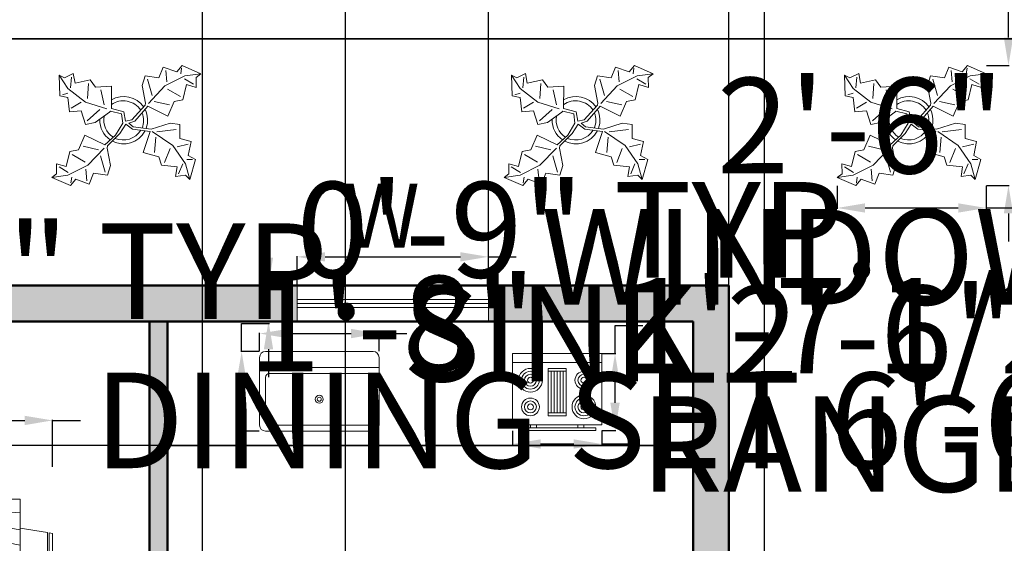
# Model space of a CAD drawing. Units: inches. Extents: x -166 to 1001, y 0 to 688.
# Tile 9 of 11: x 361 to 608, y 419 to 551. Entities that reach past the tile are written whole.
import ezdxf

# ---------------------------------------------------------------- set-up
doc = ezdxf.new("R2010")
doc.units = ezdxf.units.IN
doc.header["$MEASUREMENT"] = 0
for name, color, linetype, lineweight in [('A-ANNO-DIMS', 1, 'Continuous', 18), ('A-ANNO-TEXT', 2, 'Continuous', 25), ('A-EQPM', 11, 'Continuous', 18), ('A-FLOR-CASE', 32, 'Continuous', 25), ('A-FLOR-FIXT', 11, 'Continuous', 18), ('A-GLAZ', 130, 'Continuous', 18), ('A-WALL-PATT', 5, 'Continuous', 13), ('C-SITE-WALL', 250, 'Continuous', 35), ('FURNITURE', 11, 'Continuous', 18), ('TREES', 80, 'Continuous', 13), ('WALLS', 250, 'Continuous', 50)]:
    doc.layers.add(name, color=color, linetype=linetype, lineweight=lineweight)
doc.styles.get("Standard").update_dxf_attribs({"font": 'arial.ttf'})
doc.dimstyles.get("Standard").update_dxf_attribs({"dimtxt": 24, "dimasz": 7, "dimexe": 0.18, "dimexo": 0.0625, "dimgap": 0.09, "dimtad": 0, "dimtih": 1, "dimtoh": 1, "dimdec": 0, "dimzin": 0, "dimdsep": 46, "dimlunit": 3, "dimtxsty": 'Standard', "dimcen": 0.09, "dimadec": 0, "dimazin": 0, "dimtfac": 1, "dimtdec": 0, "dimtofl": 0, "dimtmove": 0, "dimatfit": 3, "dimfxl": 1, "dimtolj": 1, "dimtzin": 0, "dimarcsym": 0})

# ---------------------------------------------------------------- blocks, each defined once
blk = doc.blocks.new('Sink-single - 30 in top')
blk.add_line((-15, -3.999996), (15, -3.999996))
for points in [[(-13.5, 0), (13.5, 0)], [(-15, -18.499996), (-15, -1.5)], [(15, -1.5), (15, -18.499996)], [(-13.5, -17.499996), (-13.5, -6.499996)], [(-12.5, -5.499996), (12.5, -5.499996)], [(13.5, -6.499996), (13.5, -17.499996)], [(12.5, -18.499996), (-12.5, -18.499996)], [(13.5, -19.999996), (-13.5, -19.999996)]]:
    blk.add_lwpolyline(points)
for radius in [1, 0.5]:
    blk.add_circle((0, -11.999996), radius)
for centre, radius, start, end in [((-13.5, -1.5), 1.5, 90, 180), ((13.5, -1.5), 1.5, 0, 90), ((-12.5, -6.499996), 1, 90, 180), ((12.5, -6.499996), 1, 0, 90), ((-13.5, -18.499996), 1.5, 180, 270), ((-12.5, -17.499996), 1, 180, 270), ((12.5, -17.499996), 1, 270, 0), ((13.5, -18.499996), 1.5, 270, 0)]:
    blk.add_arc(centre, radius, start, end)
blk = doc.blocks.new('Range-Oven - 30 in top')
for p, q in [((0, -3), (30, -3)), ((12, -6), (18, -6)), ((13, -20), (13, -6)), ((14, -6), (14, -20)), ((15, -20), (15, -6)), ((16, -6), (16, -20)), ((17, -20), (17, -6)), ((18, -20), (12, -20)), ((6, -24), (6, -25)), ((8, -25), (8, -24)), ((22, -25), (22, -24)), ((24, -24), (24, -25))]:
    blk.add_line(p, q)
for points in [[(0, -24), (0, 0), (30, 0), (30, -24)], [(12, -21), (12, -5), (18, -5), (18, -21)], [(2, -26), (2, -25), (28, -25), (28, -26)]]:
    blk.add_lwpolyline(points, close=True)
for centre, radius in [((6, -9), 4), ((6, -9), 3), ((24, -9), 3), ((6, -9), 2), ((6, -9), 1), ((24, -9), 2), ((24, -9), 1), ((6, -18), 3), ((6, -18), 2), ((24, -18), 4), ((24, -18), 3), ((24, -18), 2), ((6, -18), 1), ((24, -18), 1)]:
    blk.add_circle(centre, radius)
blk = doc.blocks.new('Dining Set - 36 x 72 in.')
for p, q in [((-22.2343, 26.00059), (-23.4847, 17.99762)), ((-22.2304, 26), (-5.7608, 26)), ((-22, 27.5), (-22.1562, 26.50042)), ((-5.8416, 26.5), (-22.1534, 26.5)), ((-22, 27.5), (-6, 27.5)), ((-5.8437, 26.49966), (-6, 27.5)), ((-4.5152, 17.99762), (-5.7655, 25.99926)), ((5.7657, 26.00059), (4.5153, 17.99762)), ((5.7696, 26), (22.2392, 26)), ((6, 27.5), (5.8438, 26.50042)), ((22.1584, 26.5), (5.8466, 26.5)), ((6, 27.5), (22, 27.5)), ((22.1563, 26.49966), (22, 27.5)), ((23.4848, 17.99762), (22.2345, 25.99926)), ((36, 18), (-36, 18)), ((-36, 18), (-36, -18)), ((36, -18), (36, 18)), ((-44.0006, 8.23428), (-35.9976, 9.48474)), ((44.0006, 8.23428), (35.9976, 9.48474)), ((-45.5, 8), (-44.5004, 8.15617)), ((-45.5, 8), (-45.5, -8)), ((-44.5, -8.15843), (-44.5, 8.15338)), ((-44, 8.23041), (-44, -8.23915)), ((44, 8.23041), (44, -8.23915)), ((44.5, -8.15843), (44.5, 8.15338)), ((45.5, 8), (44.5005, 8.15617)), ((45.5, 8), (45.5, -8)), ((-44.4997, -8.15631), (-45.5, -8)), ((-35.9976, -9.48476), (-43.9993, -8.2345)), ((35.9976, -9.48476), (43.9993, -8.2345)), ((44.4997, -8.15631), (45.5, -8)), ((-36, -18), (36, -18)), ((-22.2343, -26.0006), (-23.4847, -17.99762)), ((-4.5152, -17.99762), (-5.7655, -25.99928)), ((5.7657, -26.0006), (4.5153, -17.99762)), ((23.4848, -17.99762), (22.2345, -25.99928)), ((-22.2304, -26), (-5.7608, -26)), ((-22, -27.5), (-22.1562, -26.50044)), ((-5.8416, -26.5), (-22.1534, -26.5)), ((-22, -27.5), (-6, -27.5)), ((-5.8437, -26.49967), (-6, -27.5)), ((5.7696, -26), (22.2392, -26)), ((6, -27.5), (5.8438, -26.50044)), ((22.1584, -26.5), (5.8466, -26.5)), ((6, -27.5), (22, -27.5)), ((22.1563, -26.49967), (22, -27.5))]:
    blk.add_line(p, q)
for points in [[(-36, 15), (-31.1772, 14.97754), (-26.8079, 14.91406), (-22.8538, 14.81543), (-19.276, 14.6875), (-16.0362, 14.53613), (-13.0957, 14.36718), (-10.4159, 14.18652), (-7.9583, 14), (-5.6904, 13.81315), (-3.6035, 13.63021), (-1.6954, 13.45508), (0.0365, 13.29166), (1.5945, 13.14388), (2.9811, 13.01562), (4.1988, 12.9108), (5.25, 12.83333), (6.1393, 12.78613), (6.8802, 12.76823), (7.4883, 12.77767), (7.9792, 12.8125), (8.3685, 12.87077), (8.6719, 12.95052), (8.9049, 13.0498), (9.0833, 13.16666), (9.2205, 13.29899), (9.3216, 13.44401), (9.3895, 13.59879), (9.4271, 13.76041), (9.4373, 13.92594), (9.4232, 14.09245), (9.3875, 14.257), (9.3333, 14.41666), (9.2638, 14.56917), (9.1836, 14.71484), (9.0975, 14.85465), (9.0104, 14.98958), (8.9272, 15.1206), (8.8529, 15.2487), (8.7922, 15.37483), (8.75, 15.5), (8.7305, 15.62467), (8.7344, 15.74739), (8.7617, 15.86621), (8.8125, 15.97916), (8.8867, 16.08431), (8.9844, 16.17968), (9.1055, 16.26334), (9.25, 16.33333), (9.4189, 16.38802), (9.6172, 16.42708), (9.8506, 16.45052), (10.125, 16.45833), (10.4463, 16.45052), (10.8203, 16.42708), (11.2529, 16.38802), (11.75, 16.33333), (12.3184, 16.26318), (12.9694, 16.17838), (13.7151, 16.07991), (14.5677, 15.96875), (15.5395, 15.84586), (16.6426, 15.71224), (17.8893, 15.56884), (19.2917, 15.41666), (20.859, 15.25667), (22.5879, 15.08984), (24.4721, 14.91715), (26.5052, 14.73958), (28.6809, 14.5581), (30.9929, 14.3737), (33.4347, 14.18733), (36, 14)], [(-36, 10), (-28.9766, 10.14274), (-23.1725, 10.20442), (-18.4241, 10.19775), (-14.5677, 10.13541), (-11.4399, 10.03011), (-8.877, 9.89453), (-6.7154, 9.74137), (-4.7917, 9.58333), (-2.9698, 9.43082), (-1.2246, 9.28515), (0.4415, 9.14534), (2.026, 9.01041), (3.5266, 8.87939), (4.9408, 8.7513), (6.266, 8.62516), (7.5, 8.5), (8.6411, 8.37549), (9.6914, 8.2539), (10.6538, 8.13818), (11.5312, 8.03125), (12.3267, 7.93603), (13.043, 7.85547), (13.6831, 7.79248), (14.25, 7.75), (14.7471, 7.7303), (15.1797, 7.73307), (15.5537, 7.75732), (15.875, 7.80208), (16.1494, 7.86637), (16.3828, 7.94922), (16.5811, 8.04964), (16.75, 8.16666), (16.8944, 8.29915), (17.0143, 8.44531), (17.1089, 8.60319), (17.1771, 8.77083), (17.218, 8.94629), (17.2305, 9.1276), (17.2137, 9.31282), (17.1667, 9.5), (17.0895, 9.6875), (16.987, 9.875), (16.8649, 10.0625), (16.7292, 10.25), (16.5856, 10.4375), (16.4401, 10.625), (16.2985, 10.8125), (16.1667, 11), (16.05, 11.18733), (15.9518, 11.3737), (15.8752, 11.5581), (15.8229, 11.73958), (15.798, 11.91715), (15.8034, 12.08984), (15.842, 12.25667), (15.9167, 12.41666), (16.0295, 12.56836), (16.1784, 12.70833), (16.3605, 12.83268), (16.5729, 12.9375), (16.8127, 13.01888), (17.0768, 13.07291), (17.3625, 13.0957), (17.6667, 13.08333), (17.9894, 13.03312), (18.3418, 12.94726), (18.7382, 12.82918), (19.1927, 12.68229), (19.7195, 12.51001), (20.3327, 12.31575), (21.0465, 12.10294), (21.875, 11.875), (22.8357, 11.63354), (23.959, 11.37304), (25.2786, 11.08618), (26.8282, 10.76562), (28.6414, 10.40405), (30.752, 9.99414), (33.1936, 9.52856), (36, 9)], [(-36, 5.5), (-30.7157, 5.3348), (-26.069, 5.20963), (-21.9946, 5.11767), (-18.4271, 5.05208), (-15.3009, 5.00602), (-12.5508, 4.97265), (-10.1112, 4.94515), (-7.9167, 4.91666), (-5.909, 4.88167), (-4.0586, 4.83984), (-2.3429, 4.79215), (-0.7396, 4.73958), (0.7739, 4.6831), (2.22, 4.6237), (3.6213, 4.56233), (5, 4.5), (6.373, 4.43782), (7.7344, 4.3776), (9.0723, 4.32129), (10.375, 4.27083), (11.6309, 4.22819), (12.8281, 4.19531), (13.9551, 4.17415), (15, 4.16666), (15.954, 4.17448), (16.819, 4.19791), (17.6001, 4.23698), (18.3021, 4.29166), (18.9299, 4.36198), (19.4883, 4.44791), (19.9823, 4.54948), (20.4167, 4.66666), (20.7969, 4.79899), (21.1302, 4.94401), (21.4245, 5.09879), (21.6875, 5.26041), (21.9271, 5.42594), (22.1511, 5.59245), (22.3672, 5.757), (22.5834, 5.91666), (22.8065, 6.06868), (23.0404, 6.21093), (23.2879, 6.34147), (23.5521, 6.45833), (23.8358, 6.55957), (24.142, 6.64323), (24.4735, 6.70735), (24.8334, 6.75), (25.2235, 6.76969), (25.642, 6.76692), (26.0858, 6.74267), (26.5521, 6.69791), (27.0379, 6.63362), (27.5404, 6.55078), (28.0565, 6.45036), (28.5834, 6.33333), (29.1242, 6.19987), (29.7071, 6.04687), (30.3661, 5.87044), (31.1354, 5.66666), (32.0493, 5.43164), (33.142, 5.16146), (34.4475, 4.85221), (36, 4.5)], [(-36, -1), (-30.7915, -0.6591), (-26.0195, -0.38216), (-21.6519, -0.16284), (-17.6563, 0.00521), (-14.0005, 0.12833), (-10.6523, 0.21289), (-7.5796, 0.26522), (-4.75, 0.29166), (-2.134, 0.29793), (0.2878, 0.28711), (2.5317, 0.26163), (4.6146, 0.22396), (6.5529, 0.17651), (8.3633, 0.12174), (10.0623, 0.06209), (11.6667, 0), (13.1899, -0.06201), (14.6341, -0.1211), (15.9982, -0.17432), (17.2813, -0.21875), (18.4823, -0.25147), (19.6003, -0.26953), (20.6343, -0.27002), (21.5834, -0.25), (22.4481, -0.20768), (23.2357, -0.14584), (23.9549, -0.06836), (24.6146, 0.02083), (25.2235, 0.11784), (25.7904, 0.21875), (26.3241, 0.31966), (26.8334, 0.41666), (27.3265, 0.50618), (27.8099, 0.58593), (28.2894, 0.65397), (28.7709, 0.70833), (29.2601, 0.74707), (29.763, 0.76823), (30.2855, 0.76985), (30.8334, 0.75), (31.4088, 0.70784), (31.9994, 0.64713), (32.589, 0.57275), (33.1615, 0.48958), (33.7008, 0.4025), (34.1908, 0.3164), (34.6153, 0.23616), (34.9584, 0.16666), (35.2099, 0.11165), (35.3848, 0.07031), (35.504, 0.04069), (35.5886, 0.02083), (35.6594, 0.00879), (35.7377, 0.0026), (35.8442, 0.00032), (36, 0)], [(-36, -6.5), (-27.1843, -6.31267), (-20.084, -6.1263), (-14.469, -5.9419), (-10.1094, -5.76042), (-6.7752, -5.58285), (-4.2363, -5.41016), (-2.2629, -5.24333), (-0.625, -5.08334), (0.8708, -4.93099), (2.2715, -4.78646), (3.5872, -4.64974), (4.8281, -4.52084), (6.0046, -4.39974), (7.127, -4.28646), (8.2053, -4.18099), (9.25, -4.08334), (10.2705, -3.99382), (11.2734, -3.91407), (12.2647, -3.84603), (13.25, -3.79167), (14.2354, -3.75293), (15.2266, -3.73177), (16.2295, -3.73015), (17.25, -3.75), (18.2912, -3.79248), (19.3451, -3.85547), (20.4009, -3.93604), (21.4479, -4.03125), (22.4754, -4.13819), (23.4727, -4.25391), (24.4289, -4.37549), (25.3334, -4.5), (26.1785, -4.62492), (26.9694, -4.74935), (27.7145, -4.87281), (28.4219, -4.99479), (29.1, -5.11483), (29.7572, -5.23242), (30.4016, -5.34709), (31.0417, -5.45834), (31.6837, -5.56437), (32.3262, -5.65821), (32.9658, -5.73153), (33.599, -5.77604), (34.2224, -5.78345), (34.8327, -5.74545), (35.4264, -5.65373), (36, -5.5)], [(-36, -10), (-26.4022, -9.81299), (-18.4675, -9.62891), (-11.9839, -9.45069), (-6.7396, -9.28125), (-2.5226, -9.12354), (0.8789, -8.98047), (3.6769, -8.85498), (6.0833, -8.75), (8.2767, -8.66765), (10.3021, -8.60677), (12.1712, -8.56543), (13.8958, -8.54167), (15.4876, -8.53353), (16.9583, -8.53907), (18.3197, -8.55632), (19.5834, -8.58334), (20.7616, -8.61841), (21.8685, -8.66081), (22.9188, -8.71004), (23.9271, -8.76563), (24.9081, -8.82707), (25.8763, -8.89388), (26.8465, -8.96558), (27.8334, -9.04167), (28.8474, -9.12118), (29.8828, -9.20117), (30.93, -9.27824), (31.9792, -9.34896), (33.0205, -9.40991), (34.0443, -9.45768), (35.0407, -9.48885), (36, -9.5)], [(-36, -14.5), (-30.0881, -14.33513), (-25.0332, -14.21224), (-20.7312, -14.12647), (-17.0781, -14.07292), (-13.97, -14.04671), (-11.3027, -14.04297), (-8.9724, -14.05681), (-6.875, -14.08334), (-4.9224, -14.11833), (-3.0905, -14.16016), (-1.3709, -14.20785), (0.2448, -14.26042), (1.7647, -14.3169), (3.1973, -14.3763), (4.5507, -14.43767), (5.8333, -14.5), (7.0554, -14.5621), (8.235, -14.62175), (9.3922, -14.67652), (10.5469, -14.72396), (11.7192, -14.76164), (12.929, -14.78711), (14.1965, -14.79794), (15.5417, -14.79167), (16.9933, -14.76424), (18.6152, -14.70508), (20.4804, -14.60197), (22.6615, -14.44271), (25.2312, -14.21509), (28.2624, -13.9069), (31.8277, -13.50594), (36, -13)]]:
    blk.add_lwpolyline(points)
blk = doc.blocks.new('Plant - Rubber or Philodendron')
for p, q in [((8.8871, 10.7908), (9.9809, 13.4933)), ((9.9809, 13.4933), (13.3837, 12.301)), ((10.5828, 12.6946), (10.8893, 9.7953)), ((13.3837, 12.301), (14.68, 13.9039)), ((14.5816, 13.2037), (14.3848, 11.8033)), ((14.68, 13.9039), (19.3848, 11.8146)), ((-16.2005, 11.4774), (-13.9899, 8.1064)), ((-16.2005, 11.4774), (-14.8639, 10.7964)), ((-16.0159, 6.3329), (-16.2005, 11.4774)), ((-14.8639, 10.7964), (-12.6195, 11.8975)), ((-13.3174, 8.325), (-13.0735, 11.0065)), ((-12.6195, 11.8975), (-12.1909, 9.4345)), ((-12.1909, 9.4345), (-8.3829, 10.3)), ((-8.3829, 10.3), (-7.0549, 8.501)), ((4.6914, 8.8812), (5.3859, 11.2828)), ((5.3859, 11.2828), (8.8871, 10.7908)), ((5.9878, 10.4842), (7.1971, 6.3869)), ((15.3859, 11.3055), (10.3916, 8.7942)), ((15.2875, 10.6053), (17.5907, 9.2105)), ((19.3848, 11.8146), (15.3859, 11.3055)), ((19.3848, 11.8146), (18.1868, 10.9119)), ((18.1868, 10.9119), (18.1925, 8.4119)), ((-13.9899, 8.1064), (-9.5434, 4.7185)), ((-8.8369, 9.409), (-9.0894, 5.6095)), ((-7.0549, 8.501), (-3.0284, 8.6941)), ((-4.8529, 4.012), (-5.7184, 7.82)), ((-3.0284, 8.6941), (-3.0709, 3.1041)), ((4.6914, 8.8812), (5.5014, 4.4831)), ((10.3916, 8.7942), (6.2847, 4.4028)), ((14.2977, 6.1031), (10.9934, 7.9956)), ((15.7909, 9.1065), (14.8995, 5.3044)), ((18.1925, 8.4119), (15.7909, 9.1065)), ((-14.0069, 5.8704), (-16.0159, 6.3329)), ((-15.3434, 6.5514), (-13.9984, 6.9884)), ((-13.5868, 2.2894), (-14.0069, 5.8704)), ((14.8995, 5.3044), (12.7005, 4.8994)), ((-10.6784, 2.491), (-13.5868, 2.2894)), ((-13.1329, 3.1804), (-10.6614, 4.727)), ((-9.5858, -0.8715), (-10.6784, 2.491)), ((-9.5434, 4.7185), (-4.1917, 2.9888)), ((-9.1318, 0.0195), (-5.9793, 2.9025)), ((-3.0709, 3.1041), (0.0797, 2.3163)), ((2.1141, 0.2298), (5.4346, 3.9146)), ((6.1032, 3.6844), (2.8262, -0.031)), ((5.4346, 3.9146), (5.5014, 4.4831)), ((11.1089, 1.1958), (6.1032, 3.6844)), ((7.7005, 4.8881), (11.5025, 3.9967)), ((12.7005, 4.8994), (11.1089, 1.1958)), ((-7.1228, -0.443), (-3.5248, 2.2131)), ((-3.5248, 2.2131), (-3.3011, 2.4355)), ((-3.3011, 2.4355), (-0.5306, 1.7947)), ((-0.5306, 1.7947), (-0.2255, -0.5527)), ((-0.5306, 1.7947), (-0.5306, 1.7947)), ((0.0797, 2.3163), (0.4866, -0.031)), ((0.4866, -0.031), (2.1141, 0.2298)), ((-7.1228, -0.443), (-9.5858, -0.8715)), ((-2.019, -3.6148), (-0.2255, -0.5527)), ((-0.9375, -3.1608), (0.5883, -0.8135)), ((0.5883, -0.8135), (2.2447, -2.0916)), ((2.8262, -0.031), (1.3003, -0.5527)), ((1.3003, -0.5527), (2.4193, -1.4655)), ((2.2447, -2.0916), (6.7108, -2.6626)), ((2.4193, -1.4655), (6.895, -2.1175)), ((11.6605, -0.5413), (6.895, -2.1175)), ((8.3544, -2.7453), (13.1973, -2.1704)), ((11.6605, -0.5413), (14.1354, -0.8948)), ((14.1354, -0.8948), (14.1354, -4.4304)), ((-11.3237, -7.2629), (-9.7321, -3.5593)), ((-9.7321, -3.5593), (-4.7264, -6.0479)), ((-2.019, -3.6148), (-4.7264, -6.0479)), ((-4.0579, -6.2781), (-0.9375, -3.1608)), ((4.943, -7.9659), (6.7108, -2.6626)), ((12.3677, -6.1981), (7.219, -2.6772)), ((8.125, -4.0768), (7.7715, -7.9659)), ((14.1354, -4.4304), (16.9638, -5.1375)), ((-13.5228, -7.6679), (-11.3237, -7.2629)), ((-6.3237, -7.2516), (-10.1257, -6.3602)), ((-9.0148, -11.1577), (-4.9047, -6.8122)), ((-4.1246, -6.8466), (-4.0579, -6.2781)), ((-3.3146, -11.2447), (-4.1246, -6.8466)), ((10.2463, -10.4408), (11.6605, -6.9053)), ((15.5496, -10.7943), (12.3677, -6.1981)), ((16.2567, -5.8446), (13.4283, -6.5517)), ((16.9638, -5.1375), (16.2567, -8.673)), ((-14.4141, -11.4699), (-13.5228, -7.6679)), ((-12.921, -8.4665), (-9.6166, -10.359)), ((-4.611, -12.8477), (-5.8203, -8.7504)), ((8.8321, -9.0266), (4.943, -7.9659)), ((9.5392, -11.1479), (8.8321, -9.0266)), ((17.3174, -9.7337), (15.9032, -9.7337)), ((16.2567, -8.673), (18.0245, -9.7337)), ((18.0245, -9.7337), (16.6103, -14.6834)), ((-16.8157, -10.7754), (-14.4141, -11.4699)), ((-16.8101, -13.2754), (-16.8157, -10.7754)), ((-13.9107, -12.9688), (-16.2139, -11.574)), ((-14.0091, -13.669), (-9.0148, -11.1577)), ((-9.206, -15.0581), (-9.5126, -12.1588)), ((-3.3146, -11.2447), (-4.0092, -13.6463)), ((13.4283, -11.5015), (9.5392, -11.1479)), ((13.0748, -13.9763), (13.4283, -11.5015)), ((14.8425, -10.7943), (13.7819, -13.2692)), ((16.6103, -14.6834), (15.5496, -10.7943)), ((-18.008, -14.1781), (-16.8101, -13.2754)), ((-18.008, -14.1781), (-14.0091, -13.669)), ((-13.3032, -16.2674), (-18.008, -14.1781)), ((-12.0069, -14.6645), (-13.3032, -16.2674)), ((-13.2048, -15.5672), (-13.008, -14.1668)), ((-8.6042, -15.8568), (-12.0069, -14.6645)), ((-7.5103, -13.1543), (-8.6042, -15.8568)), ((-4.0092, -13.6463), (-7.5103, -13.1543)), ((15.5496, -13.6228), (13.0748, -13.9763)), ((16.6103, -14.6834), (15.5496, -13.6228))]:
    blk.add_line(p, q)
for centre, radius, start, end in [((0, 0), 6.1275, 34.37569, 120.1028), ((-0.0601, -0.2075), 5.2461, 33.82192, 124.9414), ((-0.098, 0.1364), 6.1288, 341.2017, 26.09184), ((0.0308, 0.1664), 6, 178.6147, 235.1169), ((0.0308, 0.1664), 5, 168.1647, 238.6725), ((-0.2664, 0.1682), 5.2775, 338.4094, 20.03007), ((-0.1102, 0.4886), 5.2883, 247.3711, 327.472), ((-0.0234, 0.3825), 6.1492, 242.5812, 331.2714)]:
    blk.add_arc(centre, radius, start, end)
blk = doc.blocks.new('WIN-48IN')
for p, q in [((0, 4.5), (0, 9)), ((0, 9), (0, 0)), ((48, 9), (48, 0)), ((0, 5.5), (48, 5.5)), ((0, 4.5), (48, 4.5)), ((0, 3.5), (48, 3.5))]:
    blk.add_line(p, q)
blk = doc.blocks.new('*D15')
at = {"layer": 'A-ANNO-DIMS', "color": 0, "lineweight": -2, "transparency": 16777216}
for p, q in [((566.06, 508.76), (566.06, 503.04)), ((603.45, 508.76), (603.45, 503.04)), ((573.06, 503.22), (596.45, 503.22)), ((603.45, 503.22), (610.45, 503.22))]:
    blk.add_line(p, q, dxfattribs=at)
at = {"layer": 'A-ANNO-DIMS', "color": 0, "transparency": 16777216}
for points in [[(573.06, 504.38), (573.06, 502.05), (566.06, 503.22)], [(596.45, 504.38), (596.45, 502.05), (603.45, 503.22)]]:
    blk.add_solid(points, dxfattribs=at)
at = {"layer": 'Defpoints', "color": 0, "transparency": 16777216}
for p in [(566.06, 508.83), (603.45, 508.83), (603.45, 503.22)]:
    blk.add_point(p, dxfattribs=at)
at = {"layer": 'A-ANNO-DIMS', "color": 0, "transparency": 16777216, "insert": (774.93, 503.22), "char_height": 24, "attachment_point": 5}
blk.add_mtext('\\A1;SHRUB 3\'-1 1/2" TYP.', dxfattribs=at)
blk = doc.blocks.new('*D16')
at = {"layer": 'A-ANNO-DIMS', "color": 0, "lineweight": -2, "transparency": 16777216}
for p, q in [((609.06, 546), (609.06, 553)), ((603.51, 539), (609.24, 539)), ((603.51, 508.83), (609.24, 508.83)), ((609.06, 501.83), (609.06, 494.83))]:
    blk.add_line(p, q, dxfattribs=at)
at = {"layer": 'A-ANNO-DIMS', "color": 0, "transparency": 16777216}
for points in [[(607.89, 546), (610.23, 546), (609.06, 539)], [(607.89, 501.83), (610.23, 501.83), (609.06, 508.83)]]:
    blk.add_solid(points, dxfattribs=at)
at = {"layer": 'Defpoints', "color": 0, "transparency": 16777216}
for p in [(603.45, 539), (609.06, 539), (603.45, 508.83)]:
    blk.add_point(p, dxfattribs=at)
at = {"layer": 'A-ANNO-DIMS', "color": 0, "transparency": 16777216, "insert": (609.06, 523.91), "char_height": 24, "attachment_point": 5}
blk.add_mtext('\\A1;2\'-6" TYP.', dxfattribs=at)
blk = doc.blocks.new('*D17')
at = {"layer": 'A-ANNO-DIMS', "color": 0, "lineweight": -2, "transparency": 16777216}
for p, q in [((430.46, 483.8), (430.46, 491.12)), ((437.46, 490.94), (471.46, 490.94)), ((478.46, 483.8), (478.46, 491.12)), ((478.46, 490.94), (485.46, 490.94))]:
    blk.add_line(p, q, dxfattribs=at)
at = {"layer": 'A-ANNO-DIMS', "color": 0, "transparency": 16777216}
for points in [[(437.46, 492.11), (437.46, 489.77), (430.46, 490.94)], [(471.46, 492.11), (471.46, 489.77), (478.46, 490.94)]]:
    blk.add_solid(points, dxfattribs=at)
at = {"layer": 'Defpoints', "color": 0, "transparency": 16777216}
for p in [(478.46, 490.94), (430.46, 483.74), (478.46, 483.74)]:
    blk.add_point(p, dxfattribs=at)
at = {"layer": 'A-ANNO-DIMS', "color": 0, "transparency": 16777216, "insert": (637.4, 490.94), "char_height": 24, "attachment_point": 5}
blk.add_mtext('\\A1;WINDOW 4\'-0" TYP.', dxfattribs=at)
blk = doc.blocks.new('*D18')
at = {"layer": 'A-ANNO-DIMS', "color": 0, "lineweight": -2, "transparency": 16777216}
for p, q in [((423.26, 490.74), (423.26, 497.74)), ((423.26, 497.74), (430.26, 497.74)), ((430.4, 483.74), (423.08, 483.74)), ((430.4, 474.74), (423.08, 474.74)), ((423.26, 467.74), (423.26, 460.74))]:
    blk.add_line(p, q, dxfattribs=at)
at = {"layer": 'A-ANNO-DIMS', "color": 0, "transparency": 16777216}
for points in [[(422.09, 490.74), (424.42, 490.74), (423.26, 483.74)], [(422.09, 467.74), (424.42, 467.74), (423.26, 474.74)]]:
    blk.add_solid(points, dxfattribs=at)
at = {"layer": 'Defpoints', "color": 0, "transparency": 16777216}
for p in [(423.26, 483.74), (430.46, 483.74), (430.46, 474.74)]:
    blk.add_point(p, dxfattribs=at)
at = {"layer": 'A-ANNO-DIMS', "color": 0, "transparency": 16777216, "insert": (503.49, 497.74), "char_height": 24, "attachment_point": 5}
blk.add_mtext('\\A1;0\'-9" TYP.', dxfattribs=at)
blk = doc.blocks.new('*D19')
at = {"layer": 'A-ANNO-DIMS', "color": 0, "lineweight": -2, "transparency": 16777216}
for p, q in [((175.47, 483.8), (175.47, 487.52)), ((182.47, 487.34), (192.47, 487.34)), ((199.47, 483.8), (199.47, 487.52)), ((199.47, 487.34), (206.47, 487.34))]:
    blk.add_line(p, q, dxfattribs=at)
at = {"layer": 'A-ANNO-DIMS', "color": 0, "transparency": 16777216}
for points in [[(182.47, 488.51), (182.47, 486.17), (175.47, 487.34)], [(192.47, 488.51), (192.47, 486.17), (199.47, 487.34)]]:
    blk.add_solid(points, dxfattribs=at)
at = {"layer": 'Defpoints', "color": 0, "transparency": 16777216}
for p in [(199.47, 487.34), (175.47, 483.74), (199.47, 483.74)]:
    blk.add_point(p, dxfattribs=at)
at = {"layer": 'A-ANNO-DIMS', "color": 0, "transparency": 16777216, "insert": (329.7, 487.34), "char_height": 24, "attachment_point": 5}
blk.add_mtext('\\A1;VENT 2\'-0" TYP.', dxfattribs=at)
blk = doc.blocks.new('*D25')
at = {"layer": 'A-ANNO-DIMS', "color": 0, "lineweight": -2, "transparency": 16777216}
for p, q in [((218.36, 399.34), (218.36, 394.26)), ((251.4, 399.34), (251.4, 394.26)), ((225.36, 394.44), (244.4, 394.44)), ((251.4, 394.44), (258.4, 394.44))]:
    blk.add_line(p, q, dxfattribs=at)
at = {"layer": 'A-ANNO-DIMS', "color": 0, "transparency": 16777216}
for points in [[(225.36, 395.61), (225.36, 393.27), (218.36, 394.44)], [(244.4, 395.61), (244.4, 393.27), (251.4, 394.44)]]:
    blk.add_solid(points, dxfattribs=at)
at = {"layer": 'Defpoints', "color": 0, "transparency": 16777216}
for p in [(218.36, 399.4), (251.4, 399.4), (251.4, 394.44)]:
    blk.add_point(p, dxfattribs=at)
at = {"layer": 'A-ANNO-DIMS', "color": 0, "transparency": 16777216, "insert": (364.72, 394.44), "char_height": 24, "attachment_point": 5}
blk.add_mtext('\\A1;WC 2\'-9" TYP.', dxfattribs=at)
blk = doc.blocks.new('*D29')
at = {"layer": 'A-ANNO-DIMS', "color": 0, "lineweight": -2, "transparency": 16777216}
for p, q in [((421.01, 467.24), (421.01, 471.85)), ((428.01, 471.67), (444.01, 471.67)), ((451.01, 467.24), (451.01, 471.85)), ((451.01, 471.67), (458.01, 471.67))]:
    blk.add_line(p, q, dxfattribs=at)
at = {"layer": 'A-ANNO-DIMS', "color": 0, "transparency": 16777216}
for points in [[(428.01, 472.84), (428.01, 470.51), (421.01, 471.67)], [(444.01, 472.84), (444.01, 470.51), (451.01, 471.67)]]:
    blk.add_solid(points, dxfattribs=at)
at = {"layer": 'Defpoints', "color": 0, "transparency": 16777216}
for p in [(451.01, 471.67), (421.01, 467.17), (451.01, 467.17)]:
    blk.add_point(p, dxfattribs=at)
at = {"layer": 'A-ANNO-DIMS', "color": 0, "transparency": 16777216, "insert": (533.73, 471.67), "char_height": 24, "attachment_point": 5}
blk.add_mtext('\\A1;SINK 2\'-6"', dxfattribs=at)
blk = doc.blocks.new('*D30')
at = {"layer": 'A-ANNO-DIMS', "color": 0, "lineweight": -2, "transparency": 16777216}
for p, q in [((416.51, 467.17), (416.51, 474.17)), ((416.51, 474.17), (423.51, 474.17)), ((420.95, 467.17), (416.33, 467.17)), ((416.51, 454.17), (416.51, 460.17)), ((420.95, 447.17), (416.33, 447.17))]:
    blk.add_line(p, q, dxfattribs=at)
at = {"layer": 'A-ANNO-DIMS', "color": 0, "transparency": 16777216}
for points in [[(415.34, 460.17), (417.68, 460.17), (416.51, 467.17)], [(415.34, 454.17), (417.68, 454.17), (416.51, 447.17)]]:
    blk.add_solid(points, dxfattribs=at)
at = {"layer": 'Defpoints', "color": 0, "transparency": 16777216}
for p in [(416.51, 467.17), (421.01, 467.17), (421.01, 447.17)]:
    blk.add_point(p, dxfattribs=at)
at = {"layer": 'A-ANNO-DIMS', "color": 0, "transparency": 16777216, "insert": (454.37, 474.17), "char_height": 24, "attachment_point": 5}
blk.add_mtext('\\A1;1\'-8"', dxfattribs=at)
blk = doc.blocks.new('*D31')
at = {"layer": 'A-ANNO-DIMS', "color": 0, "lineweight": -2, "transparency": 16777216}
for p, q in [((484.56, 447.22), (484.56, 443.75)), ((506.92, 447.22), (506.92, 443.75)), ((491.56, 443.93), (499.92, 443.93)), ((506.92, 443.93), (513.92, 443.93))]:
    blk.add_line(p, q, dxfattribs=at)
at = {"layer": 'A-ANNO-DIMS', "color": 0, "transparency": 16777216}
for points in [[(491.56, 445.1), (491.56, 442.76), (484.56, 443.93)], [(499.92, 445.1), (499.92, 442.76), (506.92, 443.93)]]:
    blk.add_solid(points, dxfattribs=at)
at = {"layer": 'Defpoints', "color": 0, "transparency": 16777216}
for p in [(484.56, 447.28), (506.92, 447.28), (506.92, 443.93)]:
    blk.add_point(p, dxfattribs=at)
at = {"layer": 'A-ANNO-DIMS', "color": 0, "transparency": 16777216, "insert": (646.84, 443.93), "char_height": 24, "attachment_point": 5}
blk.add_mtext('\\A1;RANGE 1\'-10 1/2"', dxfattribs=at)
blk = doc.blocks.new('*D32')
at = {"layer": 'A-ANNO-DIMS', "color": 0, "lineweight": -2, "transparency": 16777216}
for p, q in [((510.27, 466.66), (510.27, 473.66)), ((510.27, 473.66), (517.27, 473.66)), ((506.98, 466.66), (510.45, 466.66)), ((510.27, 454.28), (510.27, 459.66)), ((506.98, 447.28), (510.45, 447.28))]:
    blk.add_line(p, q, dxfattribs=at)
at = {"layer": 'A-ANNO-DIMS', "color": 0, "transparency": 16777216}
for points in [[(509.1, 459.66), (511.44, 459.66), (510.27, 466.66)], [(509.1, 454.28), (511.44, 454.28), (510.27, 447.28)]]:
    blk.add_solid(points, dxfattribs=at)
at = {"layer": 'Defpoints', "color": 0, "transparency": 16777216}
for p in [(506.92, 466.66), (510.27, 466.66), (506.92, 447.28)]:
    blk.add_point(p, dxfattribs=at)
at = {"layer": 'A-ANNO-DIMS', "color": 0, "transparency": 16777216, "insert": (576.09, 473.66), "char_height": 24, "attachment_point": 5}
blk.add_mtext('\\A1;1\'-7 1/2"', dxfattribs=at)
blk = doc.blocks.new('*D33')
at = {"layer": 'A-ANNO-DIMS', "color": 0, "lineweight": -2, "transparency": 16777216}
for p, q in [((291.16, 438.23), (291.16, 450.03)), ((369.04, 438.23), (369.04, 450.03)), ((298.16, 449.85), (362.04, 449.85)), ((369.04, 449.85), (376.04, 449.85))]:
    blk.add_line(p, q, dxfattribs=at)
at = {"layer": 'A-ANNO-DIMS', "color": 0, "transparency": 16777216}
for points in [[(298.16, 451.02), (298.16, 448.68), (291.16, 449.85)], [(362.04, 451.02), (362.04, 448.68), (369.04, 449.85)]]:
    blk.add_solid(points, dxfattribs=at)
at = {"layer": 'Defpoints', "color": 0, "transparency": 16777216}
for p in [(369.04, 449.85), (291.16, 438.17), (369.04, 438.17)]:
    blk.add_point(p, dxfattribs=at)
at = {"layer": 'A-ANNO-DIMS', "color": 0, "transparency": 16777216, "insert": (508.03, 449.85), "char_height": 24, "attachment_point": 5}
blk.add_mtext('\\A1;DINING SET 6\'-6"', dxfattribs=at)
blk = doc.blocks.new('*D35')
at = {"layer": 'A-ANNO-DIMS', "color": 0, "lineweight": -2, "transparency": 16777216}
for p, q in [((15.38, 483.8), (15.38, 593.07)), ((22.38, 592.89), (207.38, 592.89)), ((531.88, 592.89), (346.89, 592.89)), ((538.88, 483.8), (538.88, 593.07))]:
    blk.add_line(p, q, dxfattribs=at)
at = {"layer": 'A-ANNO-DIMS', "color": 0, "transparency": 16777216}
for points in [[(22.38, 594.06), (22.38, 591.72), (15.38, 592.89)], [(531.88, 594.06), (531.88, 591.72), (538.88, 592.89)]]:
    blk.add_solid(points, dxfattribs=at)
at = {"layer": 'Defpoints', "color": 0, "transparency": 16777216}
for p in [(538.88, 592.89), (15.38, 483.74), (538.88, 483.74)]:
    blk.add_point(p, dxfattribs=at)
at = {"layer": 'A-ANNO-DIMS', "color": 0, "transparency": 16777216, "insert": (277.13, 592.89), "char_height": 24, "attachment_point": 5}
blk.add_mtext('\\A1;43\'-7 1/2"', dxfattribs=at)
blk = doc.blocks.new('*D46')
at = {"layer": 'A-ANNO-DIMS', "color": 0, "lineweight": -2, "transparency": 16777216}
for p, q in [((261.38, 474.68), (261.38, 35.41)), ((298.66, 474.68), (298.66, 35.41)), ((268.38, 35.59), (291.66, 35.59)), ((298.66, 35.59), (305.66, 35.59))]:
    blk.add_line(p, q, dxfattribs=at)
at = {"layer": 'A-ANNO-DIMS', "color": 0, "transparency": 16777216}
for points in [[(268.38, 36.76), (268.38, 34.42), (261.38, 35.59)], [(291.66, 36.76), (291.66, 34.42), (298.66, 35.59)]]:
    blk.add_solid(points, dxfattribs=at)
at = {"layer": 'Defpoints', "color": 0, "transparency": 16777216}
for p in [(261.38, 474.74), (298.66, 474.74), (298.66, 35.59)]:
    blk.add_point(p, dxfattribs=at)
at = {"layer": 'A-ANNO-DIMS', "color": 0, "transparency": 16777216, "insert": (365.61, 35.59), "char_height": 24, "attachment_point": 5}
blk.add_mtext('\\A1;3\'-1 1/2"', dxfattribs=at)
blk = doc.blocks.new('*D47')
at = {"layer": 'A-ANNO-DIMS', "color": 0, "lineweight": -2, "transparency": 16777216}
for p, q in [((478.46, 483.8), (478.46, 593.07)), ((485.46, 592.89), (531.88, 592.89)), ((538.88, 483.8), (538.88, 593.07)), ((538.88, 592.89), (545.88, 592.89))]:
    blk.add_line(p, q, dxfattribs=at)
at = {"layer": 'A-ANNO-DIMS', "color": 0, "transparency": 16777216}
for points in [[(485.46, 594.06), (485.46, 591.72), (478.46, 592.89)], [(531.88, 594.06), (531.88, 591.72), (538.88, 592.89)]]:
    blk.add_solid(points, dxfattribs=at)
at = {"layer": 'Defpoints', "color": 0, "transparency": 16777216}
for p in [(538.88, 592.89), (478.46, 483.74), (538.88, 483.74)]:
    blk.add_point(p, dxfattribs=at)
at = {"layer": 'A-ANNO-DIMS', "color": 0, "transparency": 16777216, "insert": (605.83, 592.89), "char_height": 24, "attachment_point": 5}
blk.add_mtext('\\A1;5\'-0 1/2"', dxfattribs=at)
blk = doc.blocks.new('*D57')
at = {"layer": 'A-ANNO-DIMS', "color": 0, "lineweight": -2, "transparency": 16777216}
for p, q in [((531.88, 592.89), (524.88, 592.89)), ((538.88, 335.97), (538.88, 593.07)), ((547.76, 325.77), (547.76, 593.07)), ((554.76, 592.89), (561.76, 592.89))]:
    blk.add_line(p, q, dxfattribs=at)
at = {"layer": 'A-ANNO-DIMS', "color": 0, "transparency": 16777216}
for points in [[(531.88, 594.06), (531.88, 591.72), (538.88, 592.89)], [(554.76, 594.06), (554.76, 591.72), (547.76, 592.89)]]:
    blk.add_solid(points, dxfattribs=at)
at = {"layer": 'Defpoints', "color": 0, "transparency": 16777216}
for p in [(547.76, 592.89), (538.88, 335.91), (547.76, 325.71)]:
    blk.add_point(p, dxfattribs=at)
at = {"layer": 'A-ANNO-DIMS', "color": 0, "transparency": 16777216, "insert": (593.75, 592.89), "char_height": 24, "attachment_point": 5}
blk.add_mtext('\\A1;0\'-9"', dxfattribs=at)
blk = doc.blocks.new('*D62')
at = {"layer": 'A-ANNO-DIMS', "color": 0, "lineweight": -2, "transparency": 16777216}
for p, q in [((201.55, 342.8), (201.55, 593.07)), ((208.55, 592.89), (249.88, 592.89)), ((256.88, 342.8), (256.88, 593.07)), ((256.88, 592.89), (263.88, 592.89))]:
    blk.add_line(p, q, dxfattribs=at)
at = {"layer": 'A-ANNO-DIMS', "color": 0, "transparency": 16777216}
for points in [[(208.55, 594.06), (208.55, 591.72), (201.55, 592.89)], [(249.88, 594.06), (249.88, 591.72), (256.88, 592.89)]]:
    blk.add_solid(points, dxfattribs=at)
at = {"layer": 'Defpoints', "color": 0, "transparency": 16777216}
for p in [(256.88, 592.89), (201.55, 342.74), (256.88, 342.74)]:
    blk.add_point(p, dxfattribs=at)
at = {"layer": 'A-ANNO-DIMS', "color": 0, "transparency": 16777216, "insert": (324.32, 592.89), "char_height": 24, "attachment_point": 5}
blk.add_mtext('\\A1;4\'-7 1/2"', dxfattribs=at)
blk = doc.blocks.new('*D71')
at = {"layer": 'A-ANNO-DIMS', "color": 0, "lineweight": -2, "transparency": 16777216}
for p, q in [((406.66, 278.3), (406.66, 593.07)), ((413.66, 592.89), (435.61, 592.89)), ((442.61, 278.3), (442.61, 593.07)), ((442.61, 592.89), (449.61, 592.89))]:
    blk.add_line(p, q, dxfattribs=at)
at = {"layer": 'A-ANNO-DIMS', "color": 0, "transparency": 16777216}
for points in [[(413.66, 594.06), (413.66, 591.72), (406.66, 592.89)], [(435.61, 594.06), (435.61, 591.72), (442.61, 592.89)]]:
    blk.add_solid(points, dxfattribs=at)
at = {"layer": 'Defpoints', "color": 0, "transparency": 16777216}
for p in [(442.61, 592.89), (406.66, 278.24), (442.61, 278.24)]:
    blk.add_point(p, dxfattribs=at)
at = {"layer": 'A-ANNO-DIMS', "color": 0, "transparency": 16777216, "insert": (481.59, 592.89), "char_height": 24, "attachment_point": 5}
blk.add_mtext('\\A1;3\'-0"', dxfattribs=at)
blk = doc.blocks.new('*D75')
at = {"layer": 'A-ANNO-DIMS', "color": 0, "lineweight": -2, "transparency": 16777216}
for p, q in [((-120.77, 481.74), (-120.77, 488.74)), ((529.82, 474.74), (-120.95, 474.74)), ((529.82, 443.59), (-120.95, 443.59)), ((-120.77, 436.59), (-120.77, 429.59))]:
    blk.add_line(p, q, dxfattribs=at)
at = {"layer": 'A-ANNO-DIMS', "color": 0, "transparency": 16777216}
for points in [[(-121.93, 481.74), (-119.6, 481.74), (-120.77, 474.74)], [(-121.93, 436.59), (-119.6, 436.59), (-120.77, 443.59)]]:
    blk.add_solid(points, dxfattribs=at)
at = {"layer": 'Defpoints', "color": 0, "transparency": 16777216}
for p in [(529.88, 474.74), (-120.77, 443.59), (529.88, 443.59)]:
    blk.add_point(p, dxfattribs=at)
at = {"layer": 'A-ANNO-DIMS', "color": 0, "transparency": 16777216, "insert": (-120.77, 459.16), "char_height": 24, "attachment_point": 5}
blk.add_mtext('\\A1;2\'-7"', dxfattribs=at)

msp = doc.modelspace()

# ---------------------------------------------------------------- hatches: boundary and pattern name
at = {"layer": 'A-WALL-PATT'}
h = msp.add_hatch(color=256, dxfattribs=at)
h.dxf.hatch_style = 1
h.paths.add_polyline_path([(96.05, 483.74), (15.38, 483.74), (15.38, 414.29), (24.38, 414.29), (24.38, 474.74), (96.05, 474.74)])
h.paths.add_polyline_path([(175.47, 483.74), (144.05, 483.74), (144.05, 474.74), (156.38, 474.74), (175.47, 474.74)])
h.paths.add_polyline_path([(298.66, 483.74), (199.47, 483.74), (199.47, 474.74), (256.88, 474.74), (298.66, 474.74)])
h.paths.add_polyline_path([(430.46, 483.74), (346.66, 483.74), (346.66, 474.74), (393.38, 474.74), (430.46, 474.74)])
h.paths.add_polyline_path([(261.38, 474.74), (256.88, 474.74), (256.88, 342.74), (201.55, 342.74), (201.55, 338.24), (274.49, 338.24), (274.49, 342.74), (261.38, 342.74)])
h.paths.add_polyline_path([(160.88, 474.74), (156.38, 474.74), (156.38, 342.74), (146.03, 342.74), (146.03, 338.24), (171.55, 338.24), (171.55, 342.74), (160.88, 342.74)])
h.paths.add_polyline_path([(397.88, 474.74), (393.38, 474.74), (393.38, 383.21), (397.88, 383.21)])
h.paths.add_polyline_path([(538.88, 362.18), (529.88, 362.18), (529.88, 342.74), (397.88, 342.74), (397.88, 348.69), (393.38, 348.69), (393.38, 342.74), (384.24, 342.74), (384.24, 338.24), (529.88, 338.24), (529.88, 334.73), (538.88, 334.73)])
h.paths.add_polyline_path([(538.88, 483.74), (478.46, 483.74), (478.46, 474.74), (529.88, 474.74), (529.88, 410.18), (538.88, 410.18)])
h.paths.add_polyline_path([(538.88, 298.79), (529.88, 298.79), (529.88, 278.24), (442.61, 278.24), (442.61, 273.74), (529.88, 273.74), (529.88, 221.94), (538.88, 221.94)])
h.paths.add_polyline_path([(538.88, 173.94), (529.88, 173.94), (529.88, 153.74), (393.38, 153.74), (382.23, 153.74), (382.23, 144.74), (538.88, 144.74)])
h.paths.add_polyline_path([(397.88, 164.32), (393.38, 164.32), (393.38, 153.74), (397.88, 153.74)], flags=17)
h.paths.add_polyline_path([(397.88, 273.74), (406.66, 273.74), (406.66, 278.24), (393.38, 278.24), (393.38, 273.74), (393.38, 230.24), (316.88, 230.24), (316.88, 153.74), (321.38, 153.74), (321.38, 225.74), (393.38, 225.74), (393.38, 194.32), (397.88, 194.32)])
h.paths.add_polyline_path([(358.23, 153.74), (316.88, 153.74), (284.58, 153.74), (284.58, 144.74), (358.23, 144.74)])
h.paths.add_polyline_path([(224.58, 153.74), (156.38, 153.74), (149.31, 153.74), (149.31, 144.74), (224.58, 144.74)])
h.paths.add_polyline_path([(101.31, 153.74), (24.38, 153.74), (24.38, 168.41), (15.38, 168.41), (15.38, 144.74), (101.31, 144.74)])
h.paths.add_polyline_path([(160.88, 273.74), (160.88, 278.24), (147.87, 278.24), (147.87, 273.74), (156.38, 273.74), (156.38, 153.74), (160.88, 153.74)])
h.paths.add_polyline_path([(111.92, 278.24), (100.88, 278.24), (100.88, 338.24), (110.03, 338.24), (110.03, 342.74), (24.38, 342.74), (24.38, 366.29), (15.38, 366.29), (15.38, 216.41), (24.38, 216.41), (24.38, 273.74), (44.93, 273.74), (44.93, 278.24), (24.38, 278.24), (24.38, 338.24), (96.38, 338.24), (96.38, 278.24), (74.93, 278.24), (74.93, 273.74), (111.92, 273.74)])

# ---------------------------------------------------------------- linework, layer by layer
at = {"layer": 'A-FLOR-CASE'}
msp.add_line((397.88, 443.59), (529.88, 443.59), dxfattribs=at)
at = {"layer": 'C-SITE-WALL'}
msp.add_line((-73.62, 545.74), (627.88, 545.74), dxfattribs=at)
at = {"layer": 'WALLS'}
for p, q in [((15.38, 483.74), (538.88, 483.74)), ((538.88, 144.74), (538.88, 483.74)), ((256.88, 474.74), (393.38, 474.74)), ((393.38, 342.74), (393.38, 474.74)), ((393.38, 474.74), (529.88, 474.74)), ((397.88, 383.21), (397.88, 474.74)), ((529.88, 342.74), (529.88, 474.74))]:
    msp.add_line(p, q, dxfattribs=at)

# ---------------------------------------------------------------- block references
at = {"layer": 'A-EQPM', "xscale": 0.7453560521284187, "yscale": 0.7453560521284187, "zscale": 0.7453560521284187}
msp.add_blockref('Range-Oven - 30 in top', (484.56, 466.66), dxfattribs=at)
at = {"layer": 'A-FLOR-FIXT'}
msp.add_blockref('Sink-single - 30 in top', (436.01, 467.17), dxfattribs=at)
at = {"layer": 'A-GLAZ'}
msp.add_blockref('WIN-48IN', (430.46, 474.74), dxfattribs=at)
at = {"layer": 'FURNITURE', "xscale": 0.8558305474851317, "yscale": 0.8558305474851317, "zscale": 0.8558305474851317}
msp.add_blockref('Dining Set - 36 x 72 in.', (330.1, 414.63), dxfattribs=at)
at = {"layer": 'TREES'}
for p in [(386.87, 525.09), (500.44, 525.09), (584.07, 525.09)]:
    msp.add_blockref('Plant - Rubber or Philodendron', p, dxfattribs=at)

# ---------------------------------------------------------------- texts
at = {"layer": 'A-ANNO-TEXT'}
msp.add_text('W ', height=16.096, dxfattribs=at).set_placement((441.99, 493.21))

# ---------------------------------------------------------------- dimensions: what is measured, and where the dimension line sits
at = {"layer": 'A-ANNO-DIMS'}
for base, p1, p2, picture, middle in [((538.88, 592.89), (15.38, 483.74), (538.88, 483.74), '*D35', (277.13, 592.89)), ((256.88, 592.89), (201.55, 342.74), (256.88, 342.74), '*D62', (324.32, 592.89)), ((538.88, 592.89), (478.46, 483.74), (538.88, 483.74), '*D47', (605.83, 592.89)), ((442.6082, 592.8909), (406.6614, 278.2409), (442.6082, 278.2409), '*D71', (481.589, 592.8909)), ((547.76, 592.89), (538.88, 335.91), (547.76, 325.71), '*D57', (593.75, 592.89)), ((298.66, 35.59), (261.38, 474.74), (298.66, 474.74), '*D46', (365.61, 35.59))]:
    dim = msp.add_linear_dim(base=base, p1=p1, p2=p2, dimstyle='Standard', override={"dimdec": 1, "dimlfac": 1, "dimrnd": 0, "dimzin": 1, "dimdsep": 46, "dimlunit": 4, "dimfrac": 2}, dxfattribs=at)
    dim.commit()
    dim.dimension.update_dxf_attribs({"geometry": picture, "text_midpoint": middle})
for base, p1, p2, text, picture, middle in [((603.45, 503.22), (566.06, 508.83), (603.45, 508.83), 'SHRUB <> TYP.', '*D15', (774.93, 503.22)), ((478.46, 490.94), (430.46, 483.74), (478.46, 483.74), 'WINDOW <> TYP.', '*D17', (637.4, 490.94)), ((199.47, 487.34), (175.47, 483.74), (199.47, 483.74), 'VENT <> TYP.', '*D19', (329.7, 487.34)), ((451.01, 471.67), (421.01, 467.17), (451.01, 467.17), 'SINK <>', '*D29', (533.73, 471.67)), ((369.04, 449.85), (291.16, 438.17), (369.04, 438.17), 'DINING SET <>', '*D33', (508.03, 449.85)), ((506.92, 443.93), (484.56, 447.28), (506.92, 447.28), 'RANGE <>', '*D31', (646.84, 443.93)), ((251.4, 394.44), (218.36, 399.4), (251.4, 399.4), 'WC <> TYP.', '*D25', (364.72, 394.44))]:
    dim = msp.add_linear_dim(base=base, p1=p1, p2=p2, text=text, dimstyle='Standard', override={"dimdec": 1, "dimlfac": 1, "dimrnd": 0, "dimzin": 1, "dimdsep": 46, "dimlunit": 4, "dimfrac": 2}, dxfattribs=at)
    dim.commit()
    dim.dimension.update_dxf_attribs({"geometry": picture, "text_midpoint": middle})
for base, p1, p2, picture, middle in [((609.06, 539), (603.45, 508.83), (603.45, 539), '*D16', (609.06, 523.91)), ((423.26, 483.74), (430.46, 474.74), (430.46, 483.74), '*D18', (503.49, 497.74))]:
    dim = msp.add_linear_dim(base=base, p1=p1, p2=p2, angle=90, text='<> TYP.', dimstyle='Standard', override={"dimdec": 1, "dimlfac": 1, "dimrnd": 0, "dimzin": 1, "dimdsep": 46, "dimlunit": 4, "dimfrac": 2}, dxfattribs=at)
    dim.commit()
    dim.dimension.update_dxf_attribs({"geometry": picture, "text_midpoint": middle})
for base, p1, p2, picture, middle in [((510.27, 466.66), (506.92, 447.28), (506.92, 466.66), '*D32', (576.09, 473.66)), ((416.51, 467.17), (421.01, 447.17), (421.01, 467.17), '*D30', (454.37, 474.17)), ((-120.7675, 443.5862), (529.8825, 474.7409), (529.8825, 443.5862), '*D75', (-120.7675, 459.1635))]:
    dim = msp.add_linear_dim(base=base, p1=p1, p2=p2, angle=90, dimstyle='Standard', override={"dimdec": 1, "dimlfac": 1, "dimrnd": 0, "dimzin": 1, "dimdsep": 46, "dimlunit": 4, "dimfrac": 2}, dxfattribs=at)
    dim.commit()
    dim.dimension.update_dxf_attribs({"geometry": picture, "text_midpoint": middle})

doc.saveas('drawing.dxf')
